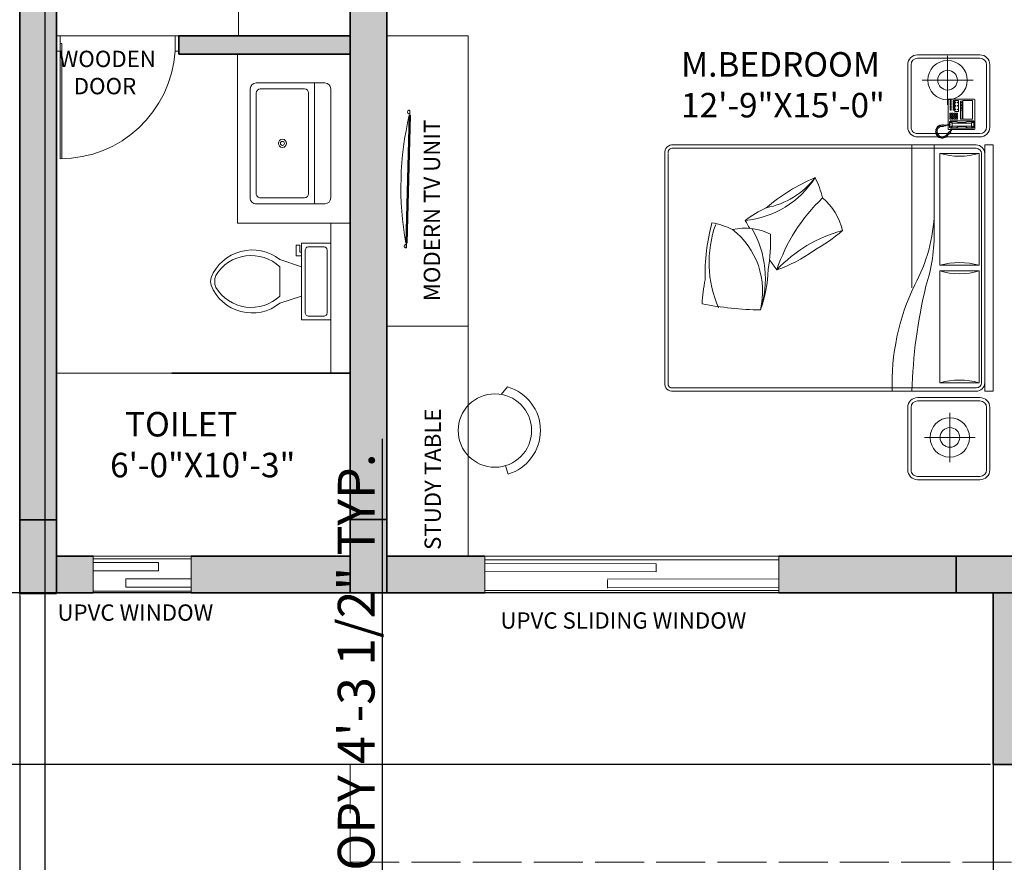
# Model space of a CAD drawing. Units: millimetres. Extents: x 595116 to 630915, y 909473 to 920225.
# Tile 119 of 134: x 629505 to 629746, y 919346 to 919552. Entities that reach past the tile are written whole.
import ezdxf

# ---------------------------------------------------------------- set-up
doc = ezdxf.new("R2010")
doc.units = ezdxf.units.MM
doc.linetypes.add('ACAD_ISO02W100', pattern=[15, 12, -3])
for name, color, linetype, lineweight in [('A-AREA-IDEN', 7, 'Continuous', 20), ('A-EQPM', 8, 'Continuous', 13), ('A-FLOR-FIXT', 9, 'Continuous', 18), ('A-FLOR-OVHD', 253, 'ACAD_ISO02W100', 13), ('A-FURN', 32, 'Continuous', 18), ('A-WALL', 1, 'Continuous', 35), ('A-WALL-PATT', 8, 'Continuous', 13), ('Column', 6, 'Continuous', 35), ('Dimension', 3, 'Continuous', 18), ('Doors', 31, 'Continuous', 20), ('Text', 7, 'Continuous', 18), ('Windows', 33, 'Continuous', 18)]:
    doc.layers.add(name, color=color, linetype=linetype, lineweight=lineweight)
doc.styles.get("Standard").update_dxf_attribs({"font": 'arial.ttf'})
doc.dimstyles.new('ISO-25', dxfattribs={"dimtxt": 9, "dimasz": 6, "dimexe": 1.25, "dimexo": 0.625, "dimtad": 1, "dimlunit": 4, "dimtxsty": 'Standard', "dimcen": 2.5, "dimadec": 0, "dimazin": 0, "dimtfac": 1, "dimtmove": 0, "dimatfit": 3, "dimfxl": 1, "dimarcsym": 0})

# ---------------------------------------------------------------- blocks, each defined once
blk = doc.blocks.new('DS')
blk.add_lwpolyline([(630069.78, 919993.92), (630069.78, 919965.68), (630069.37, 919965.68), (630069.37, 919993.91)])
for points in [[(630041.6, 919963.81), (630041.6, 919967.56), (630040.69, 919967.56), (630040.69, 919963.81)], [(630069.78, 919963.81), (630070.69, 919963.81), (630070.69, 919967.56), (630069.78, 919967.56)]]:
    blk.add_lwpolyline(points, close=True)
blk.add_arc((630069.78, 919965.69), 28.24, 89.99, 176.196)
blk = doc.blocks.new('A$C356F0359')
for p, q in [((0.4398, 1.9801), (0.0598, 1.9801)), ((0.5489, 2), (2.0492, 2)), ((0.5489, 1.9489), (0.5489, 2)), ((2.0492, 1.9489), (2.0492, 2)), ((2.5283, 1.9801), (2.1483, 1.9801)), ((-0.0002, 1.9201), (-0.0002, 1.5401)), ((0.0198, 1.9201), (0.0198, 1.5401)), ((0.4398, 1.9601), (0.0598, 1.9601)), ((0.4798, 1.5401), (0.4798, 1.9201)), ((0.4998, 1.5401), (0.4998, 1.9201)), ((2.0492, 1.9489), (0.5489, 1.9489)), ((1.998, 1.9289), (0.6001, 1.9289)), ((2.0883, 1.9201), (2.0883, 1.5401)), ((2.1083, 1.9201), (2.1083, 1.5401)), ((2.5283, 1.9601), (2.1483, 1.9601)), ((2.5683, 1.5401), (2.5683, 1.9201)), ((2.5883, 1.5401), (2.5883, 1.9201)), ((0.1539, 1.5681), (0.1539, 1.8777)), ((0.2725, 1.8879), (0.2702, 1.8856)), ((0.2702, 1.8856), (0.2702, 1.7279)), ((0.2725, 1.8879), (0.4531, 1.8879)), ((0.3913, 1.8753), (0.277, 1.8753)), ((0.277, 1.8753), (0.277, 1.8147)), ((0.3913, 1.8147), (0.3913, 1.8753)), ((0.4016, 1.8787), (0.4062, 1.8845)), ((0.4016, 1.7404), (0.4016, 1.8787)), ((0.4062, 1.881), (0.405, 1.8765)), ((0.405, 1.8765), (0.4153, 1.8662)), ((0.405, 1.8765), (0.405, 1.8456)), ((0.4062, 1.8845), (0.4405, 1.8845)), ((0.4108, 1.8833), (0.4062, 1.881)), ((0.4108, 1.8833), (0.4382, 1.8833)), ((0.4165, 1.8685), (0.4108, 1.8833)), ((0.4153, 1.8662), (0.4165, 1.8685)), ((0.4153, 1.8147), (0.4153, 1.8662)), ((0.4325, 1.8685), (0.4165, 1.8685)), ((0.4325, 1.8685), (0.4382, 1.8833)), ((0.4336, 1.8662), (0.4325, 1.8685)), ((0.4439, 1.8765), (0.4336, 1.8662)), ((0.4336, 1.8147), (0.4336, 1.8662)), ((0.4382, 1.8833), (0.4428, 1.881)), ((0.4405, 1.8845), (0.4462, 1.8787)), ((0.4428, 1.881), (0.4439, 1.8765)), ((0.4439, 1.8765), (0.4439, 1.8456)), ((0.4462, 1.8787), (0.4462, 1.7416)), ((0.4531, 1.8879), (0.4553, 1.8856)), ((0.4553, 1.8856), (0.4553, 1.7279)), ((0.5489, 1.8977), (0.5489, 0.0512)), ((0.5689, 1.8977), (0.5689, 0.0512)), ((2.0292, 0.0512), (2.0292, 1.8977)), ((2.0492, 0.0512), (2.0492, 1.8977)), ((2.3306, 1.5822), (2.3306, 1.8917)), ((0.277, 1.8147), (0.3913, 1.8147)), ((0.3913, 1.8125), (0.2816, 1.8125)), ((0.2816, 1.8125), (0.2816, 1.801)), ((0.2816, 1.801), (0.3913, 1.801)), ((0.2907, 1.8125), (0.2907, 1.801)), ((0.2999, 1.8125), (0.2999, 1.801)), ((0.309, 1.8125), (0.309, 1.801)), ((0.3182, 1.8125), (0.3182, 1.801)), ((0.3273, 1.8125), (0.3273, 1.801)), ((0.3365, 1.8125), (0.3365, 1.801)), ((0.3913, 1.801), (0.3913, 1.8125)), ((0.405, 1.8456), (0.4073, 1.8399)), ((0.4073, 1.8399), (0.4108, 1.8342)), ((0.4108, 1.8342), (0.4119, 1.8262)), ((0.4119, 1.8262), (0.4119, 1.8147)), ((0.4119, 1.793), (0.4119, 1.8147)), ((0.4153, 1.8147), (0.4153, 1.753)), ((0.4336, 1.8147), (0.4336, 1.753)), ((0.4382, 1.8342), (0.4371, 1.8262)), ((0.4371, 1.8262), (0.4371, 1.8147)), ((0.4371, 1.793), (0.4371, 1.8147)), ((0.4416, 1.8399), (0.4382, 1.8342)), ((0.4439, 1.8456), (0.4416, 1.8399)), ((0.277, 1.7885), (0.277, 1.7679)), ((0.3445, 1.7885), (0.277, 1.7885)), ((0.277, 1.7679), (0.3445, 1.7679)), ((0.2782, 1.7622), (0.2782, 1.7576)), ((0.2896, 1.7622), (0.2782, 1.7622)), ((0.2782, 1.7576), (0.2896, 1.7576)), ((0.2782, 1.745), (0.2896, 1.745)), ((0.2782, 1.7382), (0.2782, 1.745)), ((0.2885, 1.7862), (0.2885, 1.7827)), ((0.2919, 1.7862), (0.2885, 1.7862)), ((0.2885, 1.7827), (0.2919, 1.7827)), ((0.2919, 1.7736), (0.2885, 1.7736)), ((0.2885, 1.7736), (0.2885, 1.7702)), ((0.2885, 1.7702), (0.2919, 1.7702)), ((0.2896, 1.7576), (0.2896, 1.7622)), ((0.2896, 1.745), (0.2896, 1.7382)), ((0.2919, 1.7827), (0.2919, 1.7862)), ((0.2919, 1.7702), (0.2919, 1.7736)), ((0.2942, 1.7622), (0.2942, 1.7576)), ((0.3056, 1.7622), (0.2942, 1.7622)), ((0.2942, 1.7576), (0.3056, 1.7576)), ((0.2942, 1.745), (0.3056, 1.745)), ((0.2942, 1.7382), (0.2942, 1.745)), ((0.3056, 1.7576), (0.3056, 1.7622)), ((0.3056, 1.745), (0.3056, 1.7382)), ((0.3125, 1.7862), (0.309, 1.7862)), ((0.309, 1.7862), (0.309, 1.7827)), ((0.309, 1.7827), (0.3125, 1.7827)), ((0.3125, 1.7736), (0.309, 1.7736)), ((0.309, 1.7736), (0.309, 1.7702)), ((0.309, 1.7702), (0.3125, 1.7702)), ((0.3102, 1.7622), (0.3102, 1.7576)), ((0.3216, 1.7622), (0.3102, 1.7622)), ((0.3102, 1.7576), (0.3216, 1.7576)), ((0.3102, 1.745), (0.3216, 1.745)), ((0.3102, 1.7382), (0.3102, 1.745)), ((0.3125, 1.7827), (0.3125, 1.7862)), ((0.3125, 1.7702), (0.3125, 1.7736)), ((0.3216, 1.7576), (0.3216, 1.7622)), ((0.3216, 1.745), (0.3216, 1.7382)), ((0.3376, 1.7622), (0.3262, 1.7622)), ((0.3262, 1.7622), (0.3262, 1.7576)), ((0.3262, 1.7576), (0.3376, 1.7576)), ((0.3262, 1.7382), (0.3262, 1.745)), ((0.3262, 1.745), (0.3376, 1.745)), ((0.333, 1.7862), (0.3296, 1.7862)), ((0.3296, 1.7862), (0.3296, 1.7827)), ((0.3296, 1.7827), (0.333, 1.7827)), ((0.333, 1.7736), (0.3296, 1.7736)), ((0.3296, 1.7736), (0.3296, 1.7702)), ((0.3296, 1.7702), (0.333, 1.7702)), ((0.333, 1.7827), (0.333, 1.7862)), ((0.333, 1.7702), (0.333, 1.7736)), ((0.3376, 1.7576), (0.3376, 1.7622)), ((0.3376, 1.745), (0.3376, 1.7382)), ((0.3445, 1.7679), (0.3445, 1.7885)), ((0.3548, 1.7759), (0.3548, 1.7827)), ((0.3548, 1.7827), (0.3639, 1.7827)), ((0.3639, 1.7759), (0.3548, 1.7759)), ((0.3548, 1.7633), (0.3548, 1.7702)), ((0.3548, 1.7702), (0.3639, 1.7702)), ((0.3639, 1.7633), (0.3548, 1.7633)), ((0.3548, 1.7564), (0.3639, 1.7564)), ((0.3548, 1.7496), (0.3548, 1.7564)), ((0.3639, 1.7496), (0.3548, 1.7496)), ((0.3548, 1.737), (0.3548, 1.7439)), ((0.3548, 1.7439), (0.3639, 1.7439)), ((0.3639, 1.7827), (0.3639, 1.7759)), ((0.3639, 1.7702), (0.3639, 1.7633)), ((0.3639, 1.7564), (0.3639, 1.7496)), ((0.3639, 1.7439), (0.3639, 1.737)), ((0.3685, 1.7827), (0.3776, 1.7827)), ((0.3685, 1.7759), (0.3685, 1.7827)), ((0.3776, 1.7759), (0.3685, 1.7759)), ((0.3685, 1.7633), (0.3685, 1.7702)), ((0.3685, 1.7702), (0.3776, 1.7702)), ((0.3776, 1.7633), (0.3685, 1.7633)), ((0.3685, 1.7564), (0.3776, 1.7564)), ((0.3685, 1.7496), (0.3685, 1.7564)), ((0.3776, 1.7496), (0.3685, 1.7496)), ((0.3685, 1.737), (0.3685, 1.7439)), ((0.3685, 1.7439), (0.3776, 1.7439)), ((0.3776, 1.7827), (0.3776, 1.7759)), ((0.3776, 1.7702), (0.3776, 1.7633)), ((0.3776, 1.7564), (0.3776, 1.7496)), ((0.3776, 1.7439), (0.3776, 1.737)), ((0.3822, 1.7759), (0.3822, 1.7827)), ((0.3822, 1.7827), (0.3913, 1.7827)), ((0.3913, 1.7759), (0.3822, 1.7759)), ((0.3822, 1.7633), (0.3822, 1.7702)), ((0.3822, 1.7702), (0.3913, 1.7702)), ((0.3913, 1.7633), (0.3822, 1.7633)), ((0.3822, 1.7576), (0.3913, 1.7576)), ((0.3822, 1.7507), (0.3822, 1.7576)), ((0.3913, 1.7507), (0.3822, 1.7507)), ((0.3822, 1.7439), (0.3913, 1.7439)), ((0.3822, 1.737), (0.3822, 1.7439)), ((0.3913, 1.7827), (0.3913, 1.7759)), ((0.3913, 1.7702), (0.3913, 1.7633)), ((0.3913, 1.7576), (0.3913, 1.7507)), ((0.3913, 1.7439), (0.3913, 1.737)), ((0.4073, 1.7347), (0.4016, 1.7404)), ((0.405, 1.7736), (0.4073, 1.7793)), ((0.405, 1.7427), (0.405, 1.7736)), ((0.405, 1.7427), (0.4153, 1.753)), ((0.4062, 1.7382), (0.405, 1.7427)), ((0.4073, 1.7793), (0.4108, 1.785)), ((0.4108, 1.785), (0.4119, 1.793)), ((0.4165, 1.7507), (0.4108, 1.7359)), ((0.4153, 1.753), (0.4165, 1.7507)), ((0.4325, 1.7507), (0.4165, 1.7507)), ((0.4336, 1.753), (0.4325, 1.7507)), ((0.4325, 1.7507), (0.4382, 1.7359)), ((0.4439, 1.7427), (0.4336, 1.753)), ((0.4382, 1.785), (0.4371, 1.793)), ((0.4416, 1.7793), (0.4382, 1.785)), ((0.4462, 1.7416), (0.4405, 1.7347)), ((0.4439, 1.7736), (0.4416, 1.7793)), ((0.4428, 1.7382), (0.4439, 1.7427)), ((0.4439, 1.7427), (0.4439, 1.7736)), ((0.4622, 1.7459), (0.4553, 1.7484)), ((0.4553, 1.7439), (0.4604, 1.7425)), ((0.4604, 1.7425), (0.465, 1.7388)), ((0.4654, 1.7427), (0.4622, 1.7459)), ((0.4678, 1.7405), (0.4654, 1.7427)), ((0.4721, 1.7421), (0.4678, 1.7405)), ((0.4741, 1.7401), (0.4721, 1.7421)), ((0.4725, 1.7366), (0.4741, 1.7401)), ((0.3052, 1.7226), (0.0051, 1.7226)), ((0.2702, 1.7279), (0.2725, 1.7256)), ((0.4244, 1.7256), (0.2725, 1.7256)), ((0.2896, 1.7382), (0.2782, 1.7382)), ((0.3056, 1.7382), (0.2942, 1.7382)), ((0.3216, 1.7382), (0.3102, 1.7382)), ((0.3376, 1.7382), (0.3262, 1.7382)), ((0.3639, 1.737), (0.3548, 1.737)), ((0.3776, 1.737), (0.3685, 1.737)), ((0.3913, 1.737), (0.3822, 1.737)), ((0.4108, 1.7359), (0.4062, 1.7382)), ((0.4234, 1.7347), (0.4073, 1.7347)), ((0.4108, 1.7359), (0.4234, 1.7359)), ((0.4233, 1.7393), (0.4235, 1.7294)), ((0.4268, 1.7393), (0.4233, 1.7393)), ((0.4235, 1.7294), (0.4263, 1.7179)), ((0.4263, 1.7179), (0.429, 1.707)), ((0.427, 1.697), (0.4265, 1.6915)), ((0.4265, 1.6915), (0.4332, 1.6903)), ((0.4332, 1.6903), (0.4267, 1.6864)), ((0.4267, 1.6864), (0.4272, 1.6801)), ((0.4274, 1.7301), (0.4268, 1.7393)), ((0.427, 1.7359), (0.4382, 1.7359)), ((0.4295, 1.6996), (0.427, 1.697)), ((0.4405, 1.7347), (0.4271, 1.7347)), ((0.4272, 1.6801), (0.4346, 1.6794)), ((0.429, 1.7227), (0.4274, 1.7301)), ((0.4531, 1.7256), (0.4284, 1.7256)), ((0.429, 1.707), (0.4288, 1.701)), ((0.4288, 1.701), (0.4295, 1.6996)), ((0.4318, 1.7119), (0.429, 1.7227)), ((0.4325, 1.7063), (0.4318, 1.7119)), ((0.4323, 1.7003), (0.4325, 1.7063)), ((0.4364, 1.6973), (0.4323, 1.7003)), ((0.4355, 1.6919), (0.4364, 1.6973)), ((0.4367, 1.6774), (0.4355, 1.6919)), ((0.4382, 1.7359), (0.4428, 1.7382)), ((0.4553, 1.7279), (0.4531, 1.7256)), ((0.465, 1.7388), (0.4662, 1.7372)), ((0.4662, 1.7372), (0.4686, 1.7374)), ((0.4686, 1.7374), (0.4662, 1.735)), ((0.4662, 1.735), (0.4755, 1.7268)), ((0.4753, 1.7388), (0.4725, 1.7366)), ((0.4783, 1.7356), (0.4753, 1.7388)), ((0.4755, 1.7268), (0.4906, 1.7139)), ((0.4759, 1.729), (0.4783, 1.7356)), ((0.4821, 1.7322), (0.4759, 1.729)), ((0.4874, 1.7272), (0.4821, 1.7322)), ((0.4862, 1.7199), (0.4874, 1.7272)), ((0.4914, 1.7231), (0.4862, 1.7199)), ((0.4908, 1.7135), (0.4984, 1.6917)), ((0.4958, 1.7185), (0.4914, 1.7231)), ((0.494, 1.7135), (0.4958, 1.7185)), ((0.501, 1.7142), (0.494, 1.7135)), ((0.4984, 1.6917), (0.4952, 1.6744)), ((0.4964, 1.7047), (0.5031, 1.7072)), ((0.5038, 1.7049), (0.4964, 1.7047)), ((0.5005, 1.695), (0.5054, 1.6996)), ((0.5068, 1.695), (0.5005, 1.695)), ((0.5008, 1.6871), (0.5079, 1.6892)), ((0.5068, 1.6836), (0.5008, 1.6871)), ((0.5031, 1.7072), (0.501, 1.7142)), ((0.5054, 1.6996), (0.5038, 1.7049)), ((0.5058, 1.679), (0.5068, 1.6836)), ((0.5079, 1.6892), (0.5068, 1.695)), ((2.4819, 1.7366), (2.1818, 1.7366)), ((0.4346, 1.6794), (0.4281, 1.6744)), ((0.4281, 1.6744), (0.4311, 1.669)), ((0.4311, 1.669), (0.4381, 1.6704)), ((0.4381, 1.6704), (0.4348, 1.6639)), ((0.4348, 1.6639), (0.4383, 1.6598)), ((0.4455, 1.6663), (0.4367, 1.6774)), ((0.4383, 1.6598), (0.4436, 1.6637)), ((0.4436, 1.6637), (0.4427, 1.6575)), ((0.4427, 1.6575), (0.4471, 1.6547)), ((0.4577, 1.6598), (0.4455, 1.6663)), ((0.4471, 1.6547), (0.4526, 1.6593)), ((0.4526, 1.6593), (0.4519, 1.6517)), ((0.4519, 1.6517), (0.4568, 1.6503)), ((0.4568, 1.6503), (0.4598, 1.6565)), ((0.4716, 1.6586), (0.4577, 1.6598)), ((0.4598, 1.6565), (0.4626, 1.6503)), ((0.4626, 1.6503), (0.4665, 1.6498)), ((0.4665, 1.6498), (0.4681, 1.6565)), ((0.4681, 1.6565), (0.4707, 1.6491)), ((0.4707, 1.6491), (0.4751, 1.6503)), ((0.485, 1.6644), (0.4716, 1.6586)), ((0.4751, 1.6503), (0.4753, 1.6565)), ((0.4753, 1.6565), (0.4806, 1.6519)), ((0.4806, 1.6519), (0.4843, 1.6538)), ((0.4843, 1.6538), (0.4836, 1.6607)), ((0.4836, 1.6607), (0.4885, 1.6547)), ((0.4952, 1.6744), (0.485, 1.6644)), ((0.4885, 1.6547), (0.4922, 1.6579)), ((0.4922, 1.6579), (0.4894, 1.6642)), ((0.4894, 1.6642), (0.4959, 1.6614)), ((0.4957, 1.6704), (0.5024, 1.6683)), ((0.4989, 1.6642), (0.4957, 1.6704)), ((0.4959, 1.6614), (0.4989, 1.6642)), ((0.5042, 1.673), (0.4987, 1.6792)), ((0.4987, 1.6792), (0.5058, 1.679)), ((0.5024, 1.6683), (0.5042, 1.673)), ((0.0598, 1.5001), (0.4398, 1.5001)), ((2.1483, 1.5001), (2.5283, 1.5001)), ((0.0598, 1.4801), (0.4398, 1.4801)), ((2.1483, 1.4801), (2.5283, 1.4801)), ((0.6001, 0.02), (1.998, 0.02)), ((0.6001, 0), (1.998, 0))]:
    blk.add_line(p, q)
at = {"linetype": 'ByBlock'}
for p, q in [((0.6001, 1.9147), (1.282, 1.9147)), ((0.6001, 1.6759), (0.6001, 1.9147)), ((1.282, 1.9147), (1.282, 1.6759)), ((1.3161, 1.9147), (1.998, 1.9147)), ((1.3161, 1.6759), (1.3161, 1.9147)), ((1.998, 1.9147), (1.998, 1.6759)), ((1.0687, 1.6418), (0.5489, 1.6418)), ((1.282, 1.6759), (0.6001, 1.6759)), ((1.998, 1.6759), (1.3161, 1.6759)), ((1.4185, 1.5053), (0.5489, 1.5053))]:
    blk.add_line(p, q, dxfattribs=at)
for centre in [(0.1539, 1.7226), (2.3306, 1.7366)]:
    blk.add_circle(centre, 0.12, dxfattribs=at)
for centre in [(0.1539, 1.7226), (2.3306, 1.7366)]:
    blk.add_circle(centre, 0.06)
for centre, radius, start, end in [((0.0598, 1.9201), 0.06, 90, 180), ((0.4398, 1.9201), 0.06, 0, 90), ((2.1483, 1.9201), 0.06, 90, 180), ((2.5283, 1.9201), 0.06, 0, 90), ((0.0598, 1.9201), 0.04, 90, 180), ((0.4398, 1.9201), 0.04, 0, 90), ((0.6001, 1.8977), 0.0512, 90, 180), ((0.6001, 1.8977), 0.0312, 90, 180), ((1.998, 1.8977), 0.0512, 0, 90), ((1.998, 1.8977), 0.0312, 0, 90), ((2.1483, 1.9201), 0.04, 90, 180), ((2.5283, 1.9201), 0.04, 0, 90), ((0.0598, 1.5401), 0.06, 180, 270), ((0.0598, 1.5401), 0.04, 180, 270), ((0.4398, 1.5401), 0.04, 270, 0), ((0.4398, 1.5401), 0.06, 270, 0), ((2.1483, 1.5401), 0.06, 180, 270), ((2.1483, 1.5401), 0.04, 180, 270), ((2.5283, 1.5401), 0.06, 270, 0), ((2.5283, 1.5401), 0.04, 270, 0), ((1.1471, 0.7332), 0.3575, 102.47819, 140.46254), ((1.9086, 1.3124), 0.8697, 195.33601, 226.41927), ((0.3249, 0.4335), 0.9879, 28.49711, 41.05657), ((0.9965, 0.4273), 0.548, 103.20343, 117.03623), ((1.6529, 1.7059), 1.0798, 223.63057, 251.4288), ((0.4451, 0.4375), 0.5655, 5.33912, 57.68949), ((0.4517, 0.5274), 0.4879, 10.69865, 52.68638), ((1.8195, 1.3719), 1.1652, 203.06416, 220.32086), ((0.5617, 0.4344), 0.7874, 18.35266, 36.68512), ((-0.021, 2.4319), 2.1977, 305.29657, 307.24182), ((1.5949, 0.9312), 0.734, 205.25901, 216.93514), ((1.4135, 0.487), 0.3575, 154.0418, 192.02615), ((1.3641, 0.0041), 0.6085, 71.81005, 120.13512), ((1.1372, -0.3434), 0.9879, 80.06073, 92.62018), ((1.2836, -0.1573), 0.7874, 69.91627, 88.24873), ((1.44, 0.1186), 0.4774, 76.18494, 142.00166), ((-0.6432, 0.628), 2.1977, 349.48843, 358.80544), ((-0.021, 2.4319), 2.1977, 297.92482, 299.3793), ((1.5595, 0.1789), 0.548, 154.76704, 168.59984), ((1.2647, 0.9578), 0.6885, 250.29361, 293.6414), ((1.3312, 1.4107), 1.1652, 254.62778, 271.88448), ((1.5368, 0.9609), 0.734, 256.82263, 268.49876), ((0.5943, 0.0454), 0.0458, 172.75992, 277.24008), ((0.5943, 0.0454), 0.0258, 172.75992, 277.24008), ((2.0038, 0.0454), 0.0458, 262.75992, 7.24008), ((2.0038, 0.0454), 0.0258, 262.75992, 7.24008)]:
    blk.add_arc(centre, radius, start, end)
for centre, radius, start, end in [((0.1906, 1.7953), 0.4265, 343.73979, 16.26021), ((1.6914, 1.7953), 0.4265, 163.73979, 196.26021), ((0.9067, 1.7953), 0.4265, 343.73979, 16.26021), ((2.4075, 1.7953), 0.4265, 163.73979, 196.26021), ((0.9303, 0.657), 0.9853, 61.43285, 88.12613), ((1.0826, 0.5712), 1.0706, 72.19663, 90.74184), ((2.1368, 4.5996), 3.0955, 256.42012, 268.37887), ((2.0056, 2.7745), 1.3903, 244.24266, 271.79845)]:
    blk.add_arc(centre, radius, start, end, dxfattribs=at)
blk = doc.blocks.new('Sink-single - 30 in top')
blk.add_line((-15, -3.999996), (15, -3.999996))
for points in [[(-13.5, 0), (13.5, 0)], [(-15, -18.499996), (-15, -1.5)], [(15, -1.5), (15, -18.499996)], [(-13.5, -17.499996), (-13.5, -6.499996)], [(-12.5, -5.499996), (12.5, -5.499996)], [(13.5, -6.499996), (13.5, -17.499996)], [(12.5, -18.499996), (-12.5, -18.499996)], [(13.5, -19.999996), (-13.5, -19.999996)]]:
    blk.add_lwpolyline(points)
for radius in [1, 0.5]:
    blk.add_circle((0, -11.999996), radius)
for centre, radius, start, end in [((-13.5, -1.5), 1.5, 90, 180), ((13.5, -1.5), 1.5, 0, 90), ((-12.5, -6.499996), 1, 90, 180), ((12.5, -6.499996), 1, 0, 90), ((-13.5, -18.499996), 1.5, 180, 270), ((-12.5, -17.499996), 1, 180, 270), ((12.5, -17.499996), 1, 270, 0), ((13.5, -18.499996), 1.5, 270, 0)]:
    blk.add_arc(centre, radius, start, end)
blk = doc.blocks.new('Toilet - top')
for p, q in [((9.5, -6), (9.5, -2)), ((-8, -8.5), (-8, -8)), ((-7, -8), (-7, -9.5)), ((-4, -8), (-6, -14)), ((4, -8), (6, -14)), ((-10, -8.5), (-8, -8.5)), ((-10, -9.5), (-10, -8.5)), ((-7, -9.5), (-10, -9.5)), ((4, -14), (-4, -14))]:
    blk.add_line(p, q)
blk.add_lwpolyline([(10.5, -8), (10.5, 0), (-10.5, 0), (-10.5, -8)], close=True)
for points in [[(-9.5, -2), (-9.5, -6)], [(8.5, -1), (-8.5, -1)], [(-8.5, -7), (8.5, -7)]]:
    blk.add_lwpolyline(points)
for centre, radius, start, end in [((-8.62, -1.88), 0.884, 81.8699, 188.1301), ((8.62, -1.88), 0.884, 351.8699, 98.1301), ((-8.62, -6.12), 0.884, 171.8699, 278.1301), ((8.62, -6.12), 0.884, 261.8699, 8.1301), ((3.52, -21.58), 12.17, 141.4691, 247.9714), ((4.2, -21.82), 11.33, 136.3677, 238.9468), ((-3.52, -21.58), 12.17, 292.0284, 38.5307), ((-4.2, -21.82), 11.33, 301.053, 43.6321), ((0, -27.88), 4, 245.7318, 294.2682), ((0, -29), 4, 254.8605, 285.1395)]:
    blk.add_arc(centre, radius, start, end)
blk = doc.blocks.new('TV-SCREEN')
for p, q in [((2.04, 32.58), (1.21, 1.19)), ((2.14, 32.58), (1.31, 1.19)), ((2.24, 32.58), (1.41, 1.19)), ((2.34, 32.57), (1.51, 1.18)), ((2.14, 32.58), (2.14, 33.76)), ((2.19, 32.58), (2.19, 33.76)), ((1.31, 1.19), (1.31, 0.01)), ((1.36, 1.19), (1.36, 0.01))]:
    blk.add_line(p, q)
for centre, radius, start, end in [((76.63, 14.9), 76.65, 166.662, 190.3006), ((2.09, 33.31), 0.462, 77.1755, 282.8245), ((1.26, 0.46), 0.462, 77.1755, 282.8245)]:
    blk.add_arc(centre, radius, start, end)
blk = doc.blocks.new('CHAIR-ROUND-2')
for p, q in [((12.11, 21.41), (10.53, 19.55)), ((12.22, 0), (11.59, 2.08))]:
    blk.add_line(p, q)
blk.add_circle((8.99, 10.69), 8.99)
blk.add_arc((8.99, 10.69), 11.16, 286.7943, 73.7898)
blk = doc.blocks.new('COLUMN-RECT-18X9')
h = blk.add_hatch(color=256)
h.dxf.hatch_style = 1
h.paths.add_polyline_path([(18, 9), (0, 9), (0, 0), (18, 0)])
blk.add_lwpolyline([(0, 9), (18, 9), (18, 0), (0, 0)], close=True)
blk = doc.blocks.new('COLUMN-RECT-9X18')
h = blk.add_hatch(color=256)
h.dxf.hatch_style = 1
h.paths.add_polyline_path([(9, 18), (0, 18), (0, 0), (9, 0)])
blk.add_lwpolyline([(0, 18), (9, 18), (9, 0), (0, 0)], close=True)
blk = doc.blocks.new('*D210')
at = {"layer": 'Defpoints', "color": 0, "transparency": 16777216}
for p in [(629586.23, 919310.12), (629593.95, 919310.12), (629586.23, 919258.66)]:
    blk.add_point(p, dxfattribs=at)
at = {"layer": 'Dimension', "color": 0, "lineweight": -2, "transparency": 16777216}
for p, q in [((629593.95, 919310.12), (629593.95, 919449.69)), ((629586.85, 919310.12), (629595.2, 919310.12)), ((629593.95, 919264.66), (629593.95, 919304.12)), ((629586.85, 919258.66), (629595.2, 919258.66))]:
    blk.add_line(p, q, dxfattribs=at)
at = {"layer": 'Dimension', "color": 0, "transparency": 16777216}
for points in [[(629592.95, 919304.12), (629594.95, 919304.12), (629593.95, 919310.12)], [(629592.95, 919264.66), (629594.95, 919264.66), (629593.95, 919258.66)]]:
    blk.add_solid(points, dxfattribs=at)
at = {"layer": 'Dimension', "color": 0, "transparency": 16777216, "insert": (629588.66, 919382.91), "char_height": 9, "attachment_point": 5, "rotation": 90}
blk.add_mtext('CANOPY 4\'-3 1/2" TYP.', dxfattribs=at)
blk = doc.blocks.new('*D216')
at = {"layer": 'Defpoints', "color": 0, "transparency": 16777216}
for p in [(629505.04, 919411.83), (629743.54, 919411.93), (629743.54, 918832.38)]:
    blk.add_point(p, dxfattribs=at)
at = {"layer": 'Dimension', "color": 0, "lineweight": -2, "transparency": 16777216}
for p, q in [((629505.04, 919411.2), (629505.04, 918831.13)), ((629743.54, 919411.3), (629743.54, 918831.13)), ((629511.04, 918832.38), (629737.54, 918832.38))]:
    blk.add_line(p, q, dxfattribs=at)
at = {"layer": 'Dimension', "color": 0, "transparency": 16777216}
for points in [[(629511.04, 918833.38), (629511.04, 918831.38), (629505.04, 918832.38)], [(629737.54, 918833.38), (629737.54, 918831.38), (629743.54, 918832.38)]]:
    blk.add_solid(points, dxfattribs=at)
at = {"layer": 'Dimension', "color": 0, "transparency": 16777216, "insert": (629624.29, 918837.66), "char_height": 9, "attachment_point": 5}
blk.add_mtext('19\'-10 1/2"', dxfattribs=at)
blk = doc.blocks.new('*D217')
at = {"layer": 'Defpoints', "color": 0, "transparency": 16777216}
for p in [(629743.54, 919411.93), (629155.38, 919369.93), (629743.54, 919369.93)]:
    blk.add_point(p, dxfattribs=at)
at = {"layer": 'Dimension', "color": 0, "lineweight": -2, "transparency": 16777216}
for p, q in [((629742.92, 919411.93), (629154.13, 919411.93)), ((629155.38, 919405.93), (629155.38, 919375.93)), ((629742.92, 919369.93), (629154.13, 919369.93))]:
    blk.add_line(p, q, dxfattribs=at)
at = {"layer": 'Dimension', "color": 0, "transparency": 16777216}
for points in [[(629154.38, 919405.93), (629156.38, 919405.93), (629155.38, 919411.93)], [(629154.38, 919375.93), (629156.38, 919375.93), (629155.38, 919369.93)]]:
    blk.add_solid(points, dxfattribs=at)
at = {"layer": 'Dimension', "color": 0, "transparency": 16777216, "insert": (629150.16, 919390.93), "char_height": 9, "attachment_point": 5, "rotation": 90}
blk.add_mtext('3\'-6"', dxfattribs=at)
blk = doc.blocks.new('*D220')
at = {"layer": 'Defpoints', "color": 0, "transparency": 16777216}
for p in [(629824.95, 920160.76), (629511.27, 919302.01), (629824.95, 919302.01)]:
    blk.add_point(p, dxfattribs=at)
at = {"layer": 'Dimension', "color": 0, "lineweight": -2, "transparency": 16777216}
for p, q in [((629511.27, 919302.63), (629511.27, 920162.01)), ((629824.95, 919302.63), (629824.95, 920162.01)), ((629517.27, 920160.76), (629818.95, 920160.76))]:
    blk.add_line(p, q, dxfattribs=at)
at = {"layer": 'Dimension', "color": 0, "transparency": 16777216}
for points in [[(629517.27, 920161.76), (629517.27, 920159.76), (629511.27, 920160.76)], [(629818.95, 920161.76), (629818.95, 920159.76), (629824.95, 920160.76)]]:
    blk.add_solid(points, dxfattribs=at)
at = {"layer": 'Dimension', "color": 0, "transparency": 16777216, "insert": (629668.11, 920166.03), "char_height": 9, "attachment_point": 5}
blk.add_mtext('26\'-1 1/2"', dxfattribs=at)

msp = doc.modelspace()

# ---------------------------------------------------------------- hatches: boundary and pattern name
at = {"layer": 'A-WALL-PATT'}
h = msp.add_hatch(color=256, dxfattribs=at)
h.dxf.hatch_style = 1
h.paths.add_polyline_path([(629514.041, 919591.928), (629505.041, 919591.928), (629505.041, 919429.828), (629514.041, 919429.828)])
h = msp.add_hatch(color=256, dxfattribs=at)
h.dxf.hatch_style = 1
h.paths.add_polyline_path([(629595.041, 919591.928), (629586.041, 919591.928), (629586.041, 919429.928), (629595.041, 919429.928)])
h = msp.add_hatch(color=256, dxfattribs=at)
h.dxf.hatch_style = 1
h.paths.add_polyline_path([(629586.041, 919548.428), (629544.041, 919548.428), (629544.041, 919543.928), (629586.041, 919543.928)])
h = msp.add_hatch(color=256, dxfattribs=at)
h.dxf.hatch_style = 1
h.paths.add_polyline_path([(629523.041, 919420.928), (629514.041, 919420.928), (629514.041, 919411.928), (629523.041, 919411.928)])
h = msp.add_hatch(color=256, dxfattribs=at)
h.dxf.hatch_style = 1
h.paths.add_polyline_path([(629586.041, 919420.928), (629547.041, 919420.928), (629547.041, 919411.928), (629586.041, 919411.928)])
h = msp.add_hatch(color=256, dxfattribs=at)
h.dxf.hatch_style = 1
h.paths.add_polyline_path([(629619.041, 919420.928), (629595.041, 919420.928), (629595.041, 919411.928), (629619.041, 919411.928)])
h = msp.add_hatch(color=256, dxfattribs=at)
h.dxf.hatch_style = 1
h.paths.add_polyline_path([(629734.541, 919420.928), (629691.041, 919420.928), (629691.041, 919411.928), (629734.541, 919411.928)])
h = msp.add_hatch(color=256, dxfattribs=at)
h.dxf.hatch_style = 1
h.paths.add_polyline_path([(629752.541, 919411.928), (629743.541, 919411.928), (629743.541, 919369.928), (629761.541, 919369.928), (629761.541, 919378.928), (629752.541, 919378.928)])

# ---------------------------------------------------------------- linework, layer by layer
at = {"layer": 'A-FLOR-FIXT'}
for p, q in [((629558.656, 919600.928), (629558.656, 919548.428)), ((629558.441, 919543.928), (629558.441, 919502.538)), ((629558.441, 919502.538), (629586.041, 919502.538)), ((629581.27, 919502.538), (629581.27, 919465.872)), ((629542.332, 919465.77), (629514.041, 919465.77)), ((629586.041, 919465.872), (629542.332, 919465.872)), ((629542.332, 919465.872), (629542.332, 919465.669)), ((629586.041, 919465.669), (629542.332, 919465.669))]:
    msp.add_line(p, q, dxfattribs=at)
at = {"layer": 'A-FLOR-OVHD'}
for p, q in [((629505.041, 919369.928), (629505.041, 919411.928)), ((629505.041, 919369.928), (629320.541, 919369.928)), ((629505.041, 919369.928), (629586.041, 919369.928)), ((629586.041, 919369.928), (629586.041, 919345.928)), ((629586.041, 919345.928), (629752.541, 919345.928))]:
    msp.add_line(p, q, dxfattribs=at)
at = {"layer": 'A-FURN'}
for p, q in [((629614.928, 919548.428), (629595.041, 919548.428)), ((629614.928, 919548.428), (629614.928, 919420.928)), ((629595.041, 919477.294), (629614.928, 919477.294))]:
    msp.add_line(p, q, dxfattribs=at)
at = {"layer": 'A-WALL'}
for p, q in [((629505.041, 919609.928), (629505.041, 919411.928)), ((629514.041, 919609.928), (629514.041, 919420.928)), ((629586.041, 919609.928), (629586.041, 919411.928)), ((629595.041, 919609.928), (629595.041, 919411.928)), ((629544.041, 919548.428), (629586.041, 919548.428)), ((629544.041, 919548.428), (629544.041, 919543.928)), ((629544.041, 919543.928), (629586.041, 919543.928)), ((629514.041, 919420.928), (629523.041, 919420.928)), ((629547.041, 919420.928), (629586.041, 919420.928)), ((629595.041, 919420.928), (629619.041, 919420.928)), ((629691.041, 919420.928), (629752.541, 919420.928)), ((629505.041, 919411.928), (629523.041, 919411.928)), ((629547.041, 919411.928), (629619.041, 919411.928)), ((629691.041, 919411.928), (629743.541, 919411.928)), ((629743.541, 919411.928), (629743.541, 919369.928)), ((629743.541, 919369.928), (629761.541, 919369.928))]:
    msp.add_line(p, q, dxfattribs=at)
at = {"layer": 'Doors'}
msp.add_line((629543.13, 919548.428), (629514.952, 919548.428), dxfattribs=at)
at = {"layer": 'Windows'}
for p, q in [((629523.041, 919420.928), (629523.041, 919411.928)), ((629523.041, 919420.928), (629547.041, 919420.928)), ((629523.041, 919419.357), (629539.041, 919419.357)), ((629547.041, 919420.928), (629547.041, 919411.928)), ((629619.041, 919420.928), (629619.041, 919411.928)), ((629619.041, 919420.928), (629691.041, 919420.928)), ((629619.047, 919419.165), (629661.041, 919419.079)), ((629661.041, 919419.079), (629661.041, 919417.079)), ((629691.041, 919420.928), (629691.041, 919411.928)), ((629619.043, 919417.165), (629661.041, 919417.079)), ((629649.041, 919415.357), (629691.039, 919415.271)), ((629649.041, 919415.104), (629649.041, 919413.104)), ((629523.041, 919411.928), (629547.041, 919411.928)), ((629619.041, 919411.928), (629691.041, 919411.928)), ((629649.041, 919413.357), (629691.035, 919413.271))]:
    msp.add_line(p, q, dxfattribs=at)
for points in [[(629523.041, 919420.323), (629547.041, 919420.323), (629547.041, 919412.338), (629523.041, 919412.338)], [(629619.041, 919420.035), (629691.041, 919420.035), (629691.041, 919412.508), (629619.041, 919412.508)]]:
    msp.add_lwpolyline(points, close=True, dxfattribs=at)
for points in [[(629523.041, 919417.357), (629539.041, 919417.357), (629539.041, 919419.357)], [(629547.041, 919413.357), (629531.041, 919413.357), (629531.041, 919415.357), (629547.041, 919415.357)]]:
    msp.add_lwpolyline(points, dxfattribs=at)

# ---------------------------------------------------------------- block references
at = {"layer": 'A-EQPM'}
msp.add_blockref('TV-SCREEN', (629598.47, 919496.448), dxfattribs=at)
at = {"layer": 'A-FLOR-FIXT', "rotation": 270}
for name, p, xscale, yscale, zscale in [('Sink-single - 30 in top', (629581.27, 919522.087), 0.9872623020467125, 0.9872623020467125, 0.9872623020467125), ('Toilet - top', (629581.27, 919488.247), 0.8924547258250047, 0.8924547258250047, 0.8924547258250047)]:
    msp.add_blockref(name, p, dxfattribs=dict(at, xscale=xscale, yscale=yscale, zscale=zscale))
at = {"layer": 'A-FURN', "xscale": 40.21338437233606, "yscale": 40.21338437233606, "zscale": 40.21338437233606, "rotation": 270}
msp.add_blockref('A$C356F0359', (629663.132, 919543.759), dxfattribs=at)
at = {"layer": 'A-FURN'}
msp.add_blockref('CHAIR-ROUND-2', (629612.501, 919441.023), dxfattribs=at)
at = {"layer": 'Column'}
for name, p in [('COLUMN-RECT-9X18', (629505.041, 919411.828)), ('COLUMN-RECT-9X18', (629586.041, 919411.928)), ('COLUMN-RECT-18X9', (629734.541, 919411.928))]:
    msp.add_blockref(name, p, dxfattribs=at)
at = {"layer": 'Doors', "rotation": 180}
msp.add_blockref('DS', (1259584.735, 1839512.237), dxfattribs=at)

# ---------------------------------------------------------------- texts
at = {"layer": 'A-AREA-IDEN', "char_height": 6, "attachment_point": 1}
for s, insert in [('{M.BEDROOM \\P12\'-9"X15\'-0"}', (629667.101, 919544.442)), ('{      TOILET\\P    6\'-0"X10\'-3"}', (629519.859, 919456.265))]:
    msp.add_mtext_dynamic_manual_height_columns(s, width=83.57324, gutter_width=12.5, heights=[0], dxfattribs=dict(at, insert=insert))
at = {"layer": 'Text', "char_height": 4, "attachment_point": 1}
for s, width, insert in [('{     WOODEN\\P        DOOR}', 61.33456, (629508.5, 919544.782)), ('{ UPVC WINDOW}', 61.33456, (629513.075, 919409.113)), ('{ UPVC SLIDING WINDOW}', 72.55106, (629621.61, 919407.176))]:
    msp.add_mtext_dynamic_manual_height_columns(s, width=width, gutter_width=12.5, heights=[0], dxfattribs=dict(at, insert=insert))
at = {"layer": 'Text', "char_height": 4, "attachment_point": 1, "rotation": 90}
for s, insert in [('{     MODERN TV UNIT}', (629604.054, 919477.294)), ('{     STUDY TABLE}', (629604.242, 919416.351))]:
    msp.add_mtext_dynamic_manual_height_columns(s, width=72.55106, gutter_width=12.5, heights=[0], dxfattribs=dict(at, insert=insert))

# ---------------------------------------------------------------- dimensions: what is measured, and where the dimension line sits
at = {"layer": 'Dimension'}
for base, p1, p2, picture, middle in [((629824.951, 920160.756), (629511.274, 919302.009), (629824.951, 919302.009), '*D220', (629668.113, 920166.035)), ((629743.541, 918832.378), (629505.041, 919411.828), (629743.541, 919411.928), '*D216', (629624.291, 918837.656))]:
    dim = msp.add_linear_dim(base=base, p1=p1, p2=p2, dimstyle='ISO-25', override={"dimdec": 1, "dimlfac": 1, "dimrnd": 0, "dimzin": 1, "dimdsep": 46, "dimlunit": 4, "dimfrac": 2}, dxfattribs=at)
    dim.commit()
    dim.dimension.update_dxf_attribs({"geometry": picture, "text_midpoint": middle})
dim = msp.add_linear_dim(base=(629593.946, 919310.123), p1=(629586.227, 919258.662), p2=(629586.227, 919310.123), angle=90, text='CANOPY <> TYP.', dimstyle='ISO-25', override={"dimdec": 1, "dimlfac": 1, "dimrnd": 0, "dimzin": 1, "dimdsep": 46, "dimlunit": 4, "dimfrac": 2}, dxfattribs=at)
dim.commit()
dim.dimension.update_dxf_attribs({"geometry": '*D210', "text_midpoint": (629588.662, 919382.907)})
dim = msp.add_linear_dim(base=(629155.382, 919369.928), p1=(629743.541, 919411.928), p2=(629743.541, 919369.928), angle=90, dimstyle='ISO-25', override={"dimdec": 1, "dimlfac": 1, "dimrnd": 0, "dimzin": 1, "dimdsep": 46, "dimlunit": 4, "dimfrac": 2}, dxfattribs=at)
dim.commit()
dim.dimension.update_dxf_attribs({"geometry": '*D217', "text_midpoint": (629150.159, 919390.928)})

doc.saveas('drawing.dxf')
